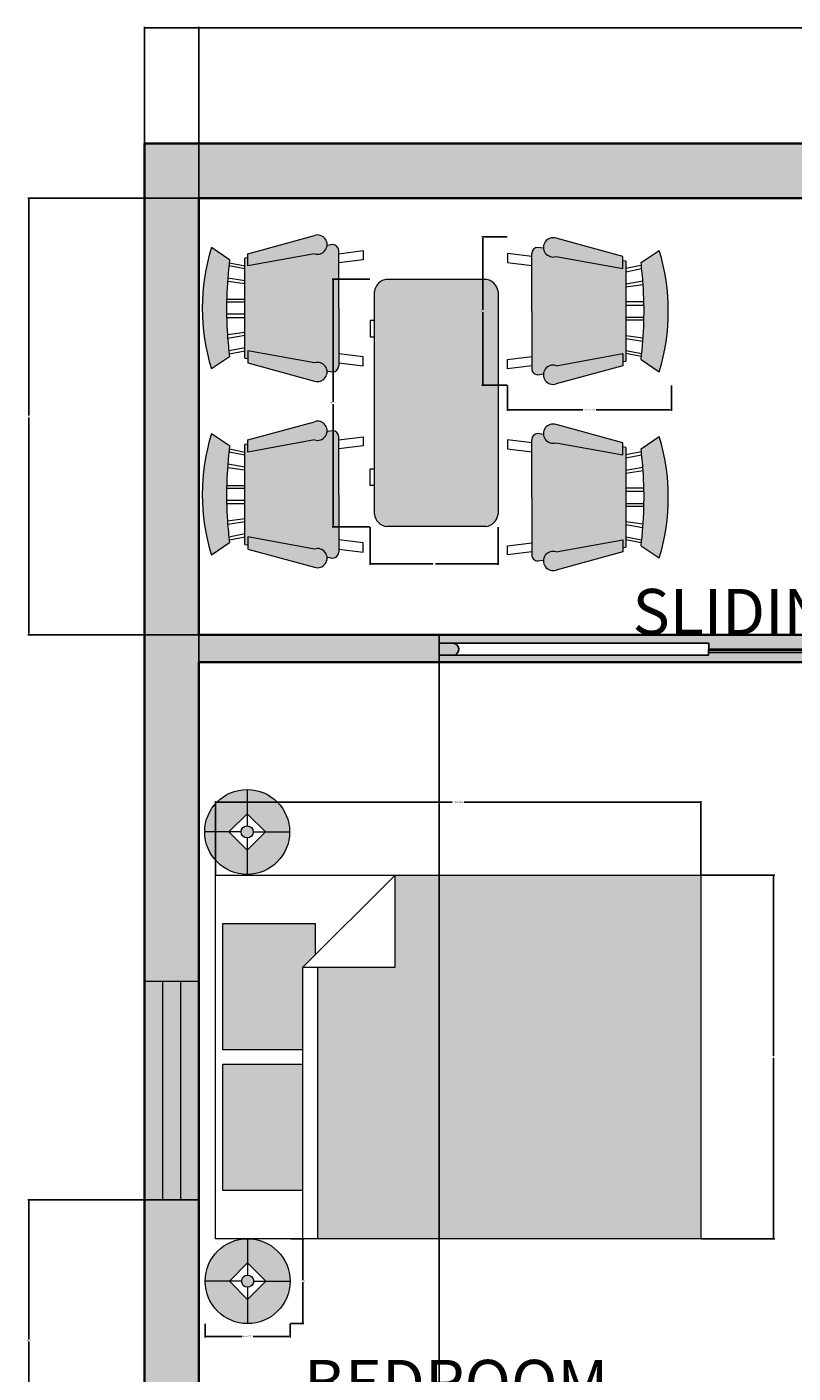
# Model space of a CAD drawing. Units: inches. Extents: x 857 to 1111, y 424 to 822.
# Tile 3 of 9: x 857 to 983, y 600 to 822. Entities that reach past the tile are written whole.
import ezdxf

# ---------------------------------------------------------------- set-up
doc = ezdxf.new("R2010")
doc.units = ezdxf.units.IN
for name, color, linetype, lineweight in [('A-ANNO-DIMS', 2, 'Continuous', 18), ('A-ANNO-TEXT', 7, 'Continuous', 18), ('A-AREA-IDEN', 7, 'Continuous', 25), ('A-DOOR', 3, 'Continuous', 25), ('A-DOOR-PATT', 17, 'Continuous', 13), ('A-FURN', 8, 'Continuous', 18), ('A-FURN-PATT', 9, 'Continuous', 13), ('A-GLAZ', 4, 'Continuous', 18), ('A-GLAZ-PATT', 9, 'Continuous', 13), ('A-WALL', 7, 'Continuous', 35), ('A-WALL-PATT', 252, 'Continuous', 13)]:
    doc.layers.add(name, color=color, linetype=linetype, lineweight=lineweight)
doc.styles.get("Standard").update_dxf_attribs({"font": 'arial.ttf'})
doc.dimstyles.get("Standard").update_dxf_attribs({"dimtxt": 0.18, "dimasz": 0.18, "dimexe": 0.18, "dimexo": 0.0625, "dimgap": 0.09, "dimtad": 0, "dimtih": 1, "dimtoh": 1, "dimdec": 4, "dimzin": 0, "dimdsep": 46, "dimtxsty": 'Standard', "dimcen": 0.09, "dimadec": 0, "dimazin": 0, "dimtfac": 1, "dimtdec": 4, "dimtofl": 0, "dimtmove": 0, "dimatfit": 3, "dimfxl": 1, "dimtolj": 1, "dimtzin": 0, "dimarcsym": 0})

# ---------------------------------------------------------------- blocks, each defined once
blk = doc.blocks.new('Bed - Queen')
for p, q in [((0, -80.00003), (0, 0)), ((0, 0), (59.99999, 0)), ((59.99999, 0), (59.99999, -80.00003)), ((7.99999, -1.2), (28.79998, -1.2)), ((7.99999, -14.4), (7.99999, -1.2)), ((28.79998, -1.2), (28.79998, -14.4)), ((31.19999, -1.2), (51.99999, -1.2)), ((31.19999, -14.4), (31.19999, -1.2)), ((51.99999, -1.2), (51.99999, -16.4)), ((0, -14.4), (44.8, -14.4)), ((59.99999, -29.6), (44.8, -14.4)), ((44.8, -14.4), (44.8, -29.6)), ((44.8, -16.8), (0, -16.8)), ((51.99999, -16.4), (46.79936, -16.4)), ((44.8, -29.6), (59.99999, -29.6)), ((59.99999, -80.00003), (0, -80.00003))]:
    blk.add_line(p, q)
blk = doc.blocks.new('Chair - Rocking')
for p, q in [((-8, -4.5), (-10, -1.5)), ((8, -4.5), (10, -1.5)), ((-6.5, -7), (-7.02225, -4.43)), ((-4.5, -7), (-4.96674, -4.19951)), ((-4, -7), (-4.40532, -4.16272)), ((-1.5, -4.05012), (-1.5, -7)), ((-1, -7), (-1, -4.05012)), ((1, -7), (1, -4.04655)), ((1.5, -4.05012), (1.5, -7)), ((4, -7), (4.40187, -4.18694)), ((4.5, -7), (4.96761, -4.19437)), ((6.5, -7), (7, -4.4057)), ((-7.5, -4.5), (-7, -7)), ((7.5, -4.5), (7, -7)), ((-9, -7.5), (-12, -18.49999)), ((-7, -7.5), (-9, -7.5)), ((-9, -18.49999), (-7, -7.5)), ((-8.23428, -6.99939), (-8.3093, -7.47958)), ((-8.23041, -7), (8.23915, -7)), ((7, -7.5), (9, -7.5)), ((9, -18.49999), (7, -7.5)), ((8.31071, -7.48854), (8.23449, -7.00073)), ((9, -7.5), (12, -18.49999)), ((-10.36644, -20.64523), (-10.5, -21.49999)), ((10.5, -21.49999), (10.3575, -20.58798)), ((-9, -22.49999), (-9.5, -26.49999)), ((0, -22.49999), (-9.5, -22.49999)), ((-8, -26.49999), (-7.5, -22.49999)), ((0, -22.49999), (9.5, -22.49999)), ((8, -26.49999), (7.5, -22.49999)), ((9, -22.49999), (9.5, -26.49999)), ((-9.5, -26.49999), (-8, -26.49999)), ((9.5, -26.49999), (8, -26.49999))]:
    blk.add_line(p, q)
for centre, radius, start, end in [((0, -34.08333), 34.08333, 72.93847, 107.0615), ((0, -68.25004), 64.25, 93.92211, 97.15267), ((0, -68.25004), 64.25, 82.84733, 93.92211), ((-10.5, -18.99999), 1.58114, 161.5651, 18.43495), ((10.5, -18.99999), 1.58114, 161.5651, 18.43495), ((-9.5, -21.49999), 1, 180, 270), ((9.5, -21.49999), 1, 270, 0)]:
    blk.add_arc(centre, radius, start, end)
blk = doc.blocks.new('Desk - 30 x 60 in.')
for p, q in [((-26.999995, 0), (26.999995, 0)), ((-29.999995, -27), (-29.999995, -3)), ((29.999995, -3), (29.999995, -27)), ((26.999995, -30), (-26.999995, -30)), ((-20.000005, -30), (-20.000005, -31)), ((-20.000005, -31), (-16.000005, -31)), ((-16.000005, -31), (-16.000005, -30)), ((15.999995, -31), (15.999995, -30)), ((19.999995, -31), (15.999995, -31)), ((19.999995, -30), (19.999995, -31))]:
    blk.add_line(p, q)
for centre, start, end in [((-26.499995, -3.5), 98.1301, 171.8699), ((26.499995, -3.5), 8.130102, 81.8699), ((-26.499995, -26.5), 188.1301, 261.8699), ((26.499995, -26.5), 278.1301, 351.8699)]:
    blk.add_arc(centre, 3.535534, start, end)
blk = doc.blocks.new('Lamp - Table')
for p, q in [((0, 7), (0, 1)), ((0, 3), (-3, 0)), ((3, 0), (0, 3)), ((-1, 0), (-7, 0)), ((-3, 0), (0, -3)), ((0, -3), (3, 0)), ((1, 0), (7, 0)), ((0, -1), (0, -7))]:
    blk.add_line(p, q)
for radius in [7, 1]:
    blk.add_circle((0, 0), radius)
blk = doc.blocks.new('WIN-36IN-9IN-WALL')
for p, q in [((3, 36), (3, 0)), ((6, 0), (6, 36))]:
    blk.add_line(p, q)
blk.add_lwpolyline([(0, 36), (0, 0), (9, 0), (9, 36)], close=True)
blk = doc.blocks.new('*D18')
at = {"layer": 'A-ANNO-DIMS', "color": 0, "lineweight": -2, "transparency": 16777216}
for p, q in [((936.02, 762.95), (936.02, 758.78)), ((963.02, 762.95), (963.02, 758.78)), ((936.2, 758.96), (948.42, 758.96)), ((962.84, 758.96), (950.62, 758.96))]:
    blk.add_line(p, q, dxfattribs=at)
at = {"layer": 'A-ANNO-DIMS', "color": 0, "transparency": 16777216}
for points in [[(936.2, 758.99), (936.2, 758.93), (936.02, 758.96)], [(962.84, 758.99), (962.84, 758.93), (963.02, 758.96)]]:
    blk.add_solid(points, dxfattribs=at)
at = {"layer": 'Defpoints', "color": 0, "transparency": 16777216}
for p in [(936.02, 763.01), (963.02, 763.01), (963.02, 758.96)]:
    blk.add_point(p, dxfattribs=at)
at = {"layer": 'A-ANNO-DIMS', "color": 0, "transparency": 16777216, "insert": (949.52, 758.96), "char_height": 0.18, "attachment_point": 5}
blk.add_mtext('\\A1;ROCKER 27 TYP.', dxfattribs=at)
blk = doc.blocks.new('*D19')
at = {"layer": 'A-ANNO-DIMS', "color": 0, "lineweight": -2, "transparency": 16777216}
for p, q in [((935.96, 787.45), (931.79, 787.45)), ((931.97, 787.27), (931.97, 775.41)), ((931.97, 763.19), (931.97, 775.05)), ((935.96, 763.01), (931.79, 763.01))]:
    blk.add_line(p, q, dxfattribs=at)
at = {"layer": 'A-ANNO-DIMS', "color": 0, "transparency": 16777216}
for points in [[(931.94, 787.27), (932, 787.27), (931.97, 787.45)], [(931.94, 763.19), (932, 763.19), (931.97, 763.01)]]:
    blk.add_solid(points, dxfattribs=at)
at = {"layer": 'Defpoints', "color": 0, "transparency": 16777216}
for p in [(936.02, 787.45), (931.97, 763.01), (936.02, 763.01)]:
    blk.add_point(p, dxfattribs=at)
at = {"layer": 'A-ANNO-DIMS', "color": 0, "transparency": 16777216, "insert": (931.97, 775.23), "char_height": 0.18, "attachment_point": 5}
blk.add_mtext('\\A1;24 TYP.', dxfattribs=at)
blk = doc.blocks.new('*D22')
at = {"layer": 'A-ANNO-DIMS', "color": 0, "lineweight": -2, "transparency": 16777216}
for p, q in [((886.16, 608.21), (886.16, 605.99)), ((900.16, 608.21), (900.16, 605.99)), ((886.34, 606.17), (892.26, 606.17)), ((899.98, 606.17), (894.06, 606.17))]:
    blk.add_line(p, q, dxfattribs=at)
at = {"layer": 'A-ANNO-DIMS', "color": 0, "transparency": 16777216}
for points in [[(886.34, 606.2), (886.34, 606.14), (886.16, 606.17)], [(899.98, 606.2), (899.98, 606.14), (900.16, 606.17)]]:
    blk.add_solid(points, dxfattribs=at)
at = {"layer": 'Defpoints', "color": 0, "transparency": 16777216}
for p in [(886.16, 608.27), (900.16, 608.27), (900.16, 606.17)]:
    blk.add_point(p, dxfattribs=at)
at = {"layer": 'A-ANNO-DIMS', "color": 0, "transparency": 16777216, "insert": (893.16, 606.17), "char_height": 0.18, "attachment_point": 5}
blk.add_mtext('\\A1;LAMP 14 TYP.', dxfattribs=at)
blk = doc.blocks.new('*D23')
at = {"layer": 'A-ANNO-DIMS', "color": 0, "lineweight": -2, "transparency": 16777216}
for p, q in [((900.23, 622.27), (902.44, 622.27)), ((902.26, 622.09), (902.26, 615.45)), ((902.26, 608.45), (902.26, 615.09)), ((900.23, 608.27), (902.44, 608.27))]:
    blk.add_line(p, q, dxfattribs=at)
at = {"layer": 'A-ANNO-DIMS', "color": 0, "transparency": 16777216}
for points in [[(902.23, 622.09), (902.29, 622.09), (902.26, 622.27)], [(902.23, 608.45), (902.29, 608.45), (902.26, 608.27)]]:
    blk.add_solid(points, dxfattribs=at)
at = {"layer": 'Defpoints', "color": 0, "transparency": 16777216}
for p in [(900.16, 622.27), (902.26, 622.27), (900.16, 608.27)]:
    blk.add_point(p, dxfattribs=at)
at = {"layer": 'A-ANNO-DIMS', "color": 0, "transparency": 16777216, "insert": (902.26, 615.27), "char_height": 0.18, "attachment_point": 5}
blk.add_mtext('\\A1;14 TYP.', dxfattribs=at)
blk = doc.blocks.new('*D28')
at = {"layer": 'A-ANNO-DIMS', "color": 0, "lineweight": -2, "transparency": 16777216}
for p, q in [((887.88, 682.29), (887.88, 694.41)), ((888.06, 694.23), (926.89, 694.23)), ((967.7, 694.23), (928.88, 694.23)), ((967.88, 682.29), (967.88, 694.41))]:
    blk.add_line(p, q, dxfattribs=at)
at = {"layer": 'A-ANNO-DIMS', "color": 0, "transparency": 16777216}
for points in [[(888.06, 694.26), (888.06, 694.2), (887.88, 694.23)], [(967.7, 694.26), (967.7, 694.2), (967.88, 694.23)]]:
    blk.add_solid(points, dxfattribs=at)
at = {"layer": 'Defpoints', "color": 0, "transparency": 16777216}
for p in [(887.88, 694.23), (887.88, 682.23), (967.88, 682.23)]:
    blk.add_point(p, dxfattribs=at)
at = {"layer": 'A-ANNO-DIMS', "color": 0, "transparency": 16777216, "insert": (927.88, 694.23), "char_height": 0.18, "attachment_point": 5}
blk.add_mtext('\\A1;QUEEN BED 80', dxfattribs=at)
blk = doc.blocks.new('*D29')
at = {"layer": 'A-ANNO-DIMS', "color": 0, "lineweight": -2, "transparency": 16777216}
for p, q in [((967.95, 682.23), (980.06, 682.23)), ((979.88, 682.05), (979.88, 652.41)), ((979.88, 622.41), (979.88, 652.04)), ((967.95, 622.23), (980.06, 622.23))]:
    blk.add_line(p, q, dxfattribs=at)
at = {"layer": 'A-ANNO-DIMS', "color": 0, "transparency": 16777216}
for points in [[(979.85, 682.05), (979.91, 682.05), (979.88, 682.23)], [(979.85, 622.41), (979.91, 622.41), (979.88, 622.23)]]:
    blk.add_solid(points, dxfattribs=at)
at = {"layer": 'Defpoints', "color": 0, "transparency": 16777216}
for p in [(967.88, 682.23), (979.88, 682.23), (967.88, 622.23)]:
    blk.add_point(p, dxfattribs=at)
at = {"layer": 'A-ANNO-DIMS', "color": 0, "transparency": 16777216, "insert": (979.88, 652.23), "char_height": 0.18, "attachment_point": 5}
blk.add_mtext('\\A1;60', dxfattribs=at)
blk = doc.blocks.new('*D42')
at = {"layer": 'A-ANNO-DIMS', "color": 0, "lineweight": -2, "transparency": 16777216}
for p, q in [((913.32, 780.49), (907.08, 780.49)), ((907.26, 780.31), (907.26, 760.27)), ((907.26, 739.86), (907.26, 759.9)), ((913.32, 739.68), (907.08, 739.68))]:
    blk.add_line(p, q, dxfattribs=at)
at = {"layer": 'A-ANNO-DIMS', "color": 0, "transparency": 16777216}
for points in [[(907.23, 780.31), (907.29, 780.31), (907.26, 780.49)], [(907.23, 739.86), (907.29, 739.86), (907.26, 739.68)]]:
    blk.add_solid(points, dxfattribs=at)
at = {"layer": 'Defpoints', "color": 0, "transparency": 16777216}
for p in [(913.38, 780.49), (907.26, 739.68), (913.38, 739.68)]:
    blk.add_point(p, dxfattribs=at)
at = {"layer": 'A-ANNO-DIMS', "color": 0, "transparency": 16777216, "insert": (907.26, 760.09), "char_height": 0.18, "attachment_point": 5}
blk.add_mtext('\\A1;DESK 41', dxfattribs=at)
blk = doc.blocks.new('*D43')
at = {"layer": 'A-ANNO-DIMS', "color": 0, "lineweight": -2, "transparency": 16777216}
for p, q in [((913.38, 739.62), (913.38, 733.38)), ((934.46, 739.62), (934.46, 733.38)), ((913.56, 733.56), (923.72, 733.56)), ((934.28, 733.56), (924.12, 733.56))]:
    blk.add_line(p, q, dxfattribs=at)
at = {"layer": 'A-ANNO-DIMS', "color": 0, "transparency": 16777216}
for points in [[(913.56, 733.59), (913.56, 733.53), (913.38, 733.56)], [(934.28, 733.59), (934.28, 733.53), (934.46, 733.56)]]:
    blk.add_solid(points, dxfattribs=at)
at = {"layer": 'Defpoints', "color": 0, "transparency": 16777216}
for p in [(913.38, 739.68), (934.46, 739.68), (934.46, 733.56)]:
    blk.add_point(p, dxfattribs=at)
at = {"layer": 'A-ANNO-DIMS', "color": 0, "transparency": 16777216, "insert": (923.92, 733.56), "char_height": 0.18, "attachment_point": 5}
blk.add_mtext('\\A1;21', dxfattribs=at)
blk = doc.blocks.new('*D44')
at = {"layer": 'A-ANNO-DIMS', "color": 0, "lineweight": -2, "transparency": 16777216}
for p, q in [((876.14, 802.92), (876.14, 822.09)), ((876.32, 821.91), (983.85, 821.91)), ((1091.96, 821.91), (984.43, 821.91)), ((1092.14, 802.92), (1092.14, 822.09))]:
    blk.add_line(p, q, dxfattribs=at)
at = {"layer": 'A-ANNO-DIMS', "color": 0, "transparency": 16777216}
for points in [[(876.32, 821.94), (876.32, 821.88), (876.14, 821.91)], [(1091.96, 821.94), (1091.96, 821.88), (1092.14, 821.91)]]:
    blk.add_solid(points, dxfattribs=at)
at = {"layer": 'Defpoints', "color": 0, "transparency": 16777216}
for p in [(1092.14, 821.91), (876.14, 802.86), (1092.14, 802.86)]:
    blk.add_point(p, dxfattribs=at)
at = {"layer": 'A-ANNO-DIMS', "color": 0, "transparency": 16777216, "insert": (984.14, 821.91), "char_height": 0.18, "attachment_point": 5}
blk.add_mtext('\\A1;216', dxfattribs=at)
blk = doc.blocks.new('*D48')
at = {"layer": 'A-ANNO-DIMS', "color": 0, "lineweight": -2, "transparency": 16777216}
for p, q in [((885.14, 582.42), (885.14, 822.09)), ((885.32, 821.91), (935, 821.91)), ((985.46, 821.91), (935.77, 821.91)), ((985.64, 582.42), (985.64, 822.09))]:
    blk.add_line(p, q, dxfattribs=at)
at = {"layer": 'A-ANNO-DIMS', "color": 0, "transparency": 16777216}
for points in [[(885.32, 821.94), (885.32, 821.88), (885.14, 821.91)], [(985.46, 821.94), (985.46, 821.88), (985.64, 821.91)]]:
    blk.add_solid(points, dxfattribs=at)
at = {"layer": 'Defpoints', "color": 0, "transparency": 16777216}
for p in [(985.64, 821.91), (885.14, 582.36), (985.64, 582.36)]:
    blk.add_point(p, dxfattribs=at)
at = {"layer": 'A-ANNO-DIMS', "color": 0, "transparency": 16777216, "insert": (935.39, 821.91), "char_height": 0.18, "attachment_point": 5}
blk.add_mtext('\\A1;100.5', dxfattribs=at)
blk = doc.blocks.new('*D54')
at = {"layer": 'A-ANNO-DIMS', "color": 0, "lineweight": -2, "transparency": 16777216}
for p, q in [((885.07, 793.86), (856.91, 793.86)), ((857.09, 793.68), (857.09, 758.04)), ((857.09, 722.04), (857.09, 757.68)), ((885.07, 721.86), (856.91, 721.86))]:
    blk.add_line(p, q, dxfattribs=at)
at = {"layer": 'A-ANNO-DIMS', "color": 0, "transparency": 16777216}
for points in [[(857.06, 793.68), (857.12, 793.68), (857.09, 793.86)], [(857.06, 722.04), (857.12, 722.04), (857.09, 721.86)]]:
    blk.add_solid(points, dxfattribs=at)
at = {"layer": 'Defpoints', "color": 0, "transparency": 16777216}
for p in [(857.09, 793.86), (885.14, 793.86), (885.14, 721.86)]:
    blk.add_point(p, dxfattribs=at)
at = {"layer": 'A-ANNO-DIMS', "color": 0, "transparency": 16777216, "insert": (857.09, 757.86), "char_height": 0.18, "attachment_point": 5}
blk.add_mtext('\\A1;72', dxfattribs=at)
blk = doc.blocks.new('*D56')
at = {"layer": 'A-ANNO-DIMS', "color": 0, "lineweight": -2, "transparency": 16777216}
for p, q in [((924.77, 717.29), (924.77, 423.63)), ((1053.97, 717.29), (1053.97, 423.63)), ((924.95, 423.81), (988.99, 423.81)), ((1053.79, 423.81), (989.75, 423.81))]:
    blk.add_line(p, q, dxfattribs=at)
at = {"layer": 'A-ANNO-DIMS', "color": 0, "transparency": 16777216}
for points in [[(924.95, 423.84), (924.95, 423.78), (924.77, 423.81)], [(1053.79, 423.84), (1053.79, 423.78), (1053.97, 423.81)]]:
    blk.add_solid(points, dxfattribs=at)
at = {"layer": 'Defpoints', "color": 0, "transparency": 16777216}
for p in [(924.77, 717.36), (1053.97, 717.36), (1053.97, 423.81)]:
    blk.add_point(p, dxfattribs=at)
at = {"layer": 'A-ANNO-DIMS', "color": 0, "transparency": 16777216, "insert": (989.37, 423.81), "char_height": 0.18, "attachment_point": 5}
blk.add_mtext('\\A1;129.2', dxfattribs=at)
blk = doc.blocks.new('*D59')
at = {"layer": 'A-ANNO-DIMS', "color": 0, "lineweight": -2, "transparency": 16777216}
for p, q in [((885.07, 628.69), (856.91, 628.69)), ((857.09, 628.51), (857.09, 605.7)), ((857.09, 582.54), (857.09, 605.34)), ((885.07, 582.36), (856.91, 582.36))]:
    blk.add_line(p, q, dxfattribs=at)
at = {"layer": 'A-ANNO-DIMS', "color": 0, "transparency": 16777216}
for points in [[(857.06, 628.51), (857.12, 628.51), (857.09, 628.69)], [(857.06, 582.54), (857.12, 582.54), (857.09, 582.36)]]:
    blk.add_solid(points, dxfattribs=at)
at = {"layer": 'Defpoints', "color": 0, "transparency": 16777216}
for p in [(857.09, 628.69), (885.14, 628.69), (885.14, 582.36)]:
    blk.add_point(p, dxfattribs=at)
at = {"layer": 'A-ANNO-DIMS', "color": 0, "transparency": 16777216, "insert": (857.09, 605.52), "char_height": 0.18, "attachment_point": 5}
blk.add_mtext('\\A1;46.33', dxfattribs=at)

msp = doc.modelspace()

# ---------------------------------------------------------------- hatches: boundary and pattern name
at = {"layer": 'A-DOOR-PATT'}
h = msp.add_hatch(color=256, dxfattribs=at)
h.dxf.hatch_style = 1
h.set_gradient(color1=(0, 0, 255), color2=(255, 255, 0))
h.paths.add_polyline_path([(1053.9717, 718.9594), (969.1676, 718.9594), (969.1596, 718.4668), (927.0274, 718.4668), (924.7696, 718.4668), (924.7696, 717.3567), (1053.9717, 717.3567)], flags=17)
h.paths.add_polyline_path([(969.1676, 718.9594), (969.1922, 720.4869), (927.0274, 720.4869, -0.93409348), (927.0274, 718.4668), (969.1596, 718.4668)], flags=0)
h.paths.add_polyline_path([(1053.9717, 721.8567), (924.7696, 721.8567), (924.7696, 720.4869), (926.8896, 720.4869, -0.03407618), (927.0274, 720.4869), (927.0302, 720.4869), (969.1922, 720.4869), (969.1759, 719.4769), (1053.9717, 719.4769)], flags=17)
h.paths.add_polyline_path([(1053.9717, 721.8567), (924.7696, 721.8567), (924.7696, 717.3567), (1053.9717, 717.3567)])
h.paths.add_polyline_path([(969.1596, 718.4668), (927.0274, 718.4668, 0.93409348), (927.0274, 720.4869), (969.1922, 720.4869)], flags=16)
h = msp.add_hatch(color=256, dxfattribs=at)
h.dxf.hatch_style = 1
h.set_gradient(color1=(0, 0, 255), color2=(255, 255, 0), name='INVCYLINDER')
h.paths.add_polyline_path([(1053.9717, 721.8567), (924.7696, 721.8567), (924.7696, 720.4869), (927.0302, 720.4869), (969.1922, 720.4869), (969.1759, 719.4769), (1053.9717, 719.4769)], flags=17)
h.paths.add_polyline_path([(1053.9717, 718.9594), (969.1676, 718.9594), (969.1759, 719.4769), (1053.9717, 719.4769), (1053.9717, 721.8567), (924.7696, 721.8567), (924.7696, 717.3567), (1053.9717, 717.3567)])
h.paths.add_polyline_path([(969.1596, 718.4668), (927.0274, 718.4668, 0.93409348), (927.0274, 720.4869), (969.1922, 720.4869)], flags=16)
h = msp.add_hatch(color=256, dxfattribs=at)
h.dxf.hatch_style = 1
h.set_gradient(color1=(0, 0, 255), color2=(255, 255, 0), name='SPHERICAL')
h.paths.add_polyline_path([(1053.9717, 721.8567), (924.7696, 721.8567), (924.7696, 717.3567), (1053.9717, 717.3567), (1053.9717, 718.9594), (969.1676, 718.9594), (969.1759, 719.4769), (1053.9717, 719.4769)])
h.paths.add_polyline_path([(927.0274, 720.4869, -0.93409348), (927.0274, 718.4668), (969.1596, 718.4668), (969.1922, 720.4869)], flags=16)
at = {"layer": 'A-FURN-PATT'}
h = msp.add_hatch(color=256, dxfattribs=at)
h.dxf.hatch_style = 1
h.paths.add_polyline_path([(967.884, 682.2251), (917.484, 682.2251), (917.484, 667.0251), (904.684, 667.0251), (904.684, 622.2251), (967.884, 622.2251)])
h.paths.add_polyline_path([(902.284, 667.0251), (904.284, 669.0251), (904.284, 674.2251), (889.084, 674.2251), (889.084, 653.4251), (902.284, 653.4251)])
h.paths.add_polyline_path([(902.284, 651.0251), (889.084, 651.0251), (889.084, 630.2251), (902.284, 630.2251)])
h.paths.add_polyline_path([(904.1909, 787.6962), (893.1909, 784.6962), (893.1909, 782.6962), (904.1909, 784.6962, 1.38742744)])
h.paths.add_polyline_path([(904.1909, 766.6962), (893.1909, 768.6962), (893.1909, 766.6962), (904.1909, 763.6962, 1.38742744)])
h.paths.add_polyline_path([(889.8414, 771.3015, -0.04836039), (890.1909, 783.6962), (887.1909, 785.6962, 0.15000001), (887.1909, 765.6962), (890.1909, 767.6962, -0.01409681)])
h.paths.add_polyline_path([(904.1909, 753.9927, 1.38742744), (904.1909, 756.9927), (893.1909, 753.9927), (893.1909, 751.9927)])
h.paths.add_polyline_path([(904.1909, 735.9927), (893.1909, 737.9927), (893.1909, 735.9927), (904.1909, 732.9927, 1.38742744)])
h.paths.add_polyline_path([(890.1909, 752.9927), (887.1909, 754.9927, 0.15000001), (887.1909, 734.9927), (890.1909, 736.9928, -0.01409681), (889.8414, 740.598, -0.04836039)])
h.paths.add_polyline_path([(955.0194, 737.5254), (944.0194, 735.5254, 1.38742744), (944.0194, 732.5254), (955.0194, 735.5254)])
h.paths.add_polyline_path([(955.0194, 753.5254), (944.0194, 756.5254, 1.38742744), (944.0194, 753.5254), (955.0194, 751.5254)])
h.paths.add_polyline_path([(955.0194, 766.2288), (955.0194, 768.2288), (944.0194, 766.2288, 1.38742744), (944.0194, 763.2288)])
h.paths.add_polyline_path([(955.0194, 784.2288), (944.0194, 787.2288, 1.38742744), (944.0194, 784.2288), (955.0194, 782.2288)])
h.paths.add_polyline_path([(961.0194, 785.2288), (958.0194, 783.2288, -0.01409681), (958.3689, 779.6235, -0.04836039), (958.0194, 767.2289), (961.0194, 765.2288, 0.15000001)])
h.paths.add_polyline_path([(961.0194, 754.5254), (958.0194, 752.5254, -0.01409681), (958.3689, 748.9201, -0.04836039), (958.0194, 736.5254), (961.0194, 734.5254, 0.15000001)])
h = msp.add_hatch(color=256, dxfattribs=at)
h.dxf.hatch_style = 1
h.paths.add_polyline_path([(908.1909, 744.9927), (908.1909, 754.4927, 0.41421356), (907.1909, 755.4927), (906.2654, 755.3481, -0.48335183), (904.1909, 753.9927), (893.1909, 751.9927), (893.1909, 753.3052), (892.6909, 753.2271), (892.6909, 736.7584), (893.1909, 736.6802), (893.1909, 737.9927), (904.1909, 735.9927, -0.4833507), (906.2654, 734.6373), (907.1909, 734.4927, 0.41421356), (908.1909, 735.4927)])
h.paths.add_polyline_path([(908.1909, 785.1962, 0.41421356), (907.1909, 786.1962), (906.2654, 786.0516, -0.48335183), (904.1909, 784.6962), (893.1909, 782.6962), (893.1909, 784.0087), (892.6909, 783.9306), (892.6909, 767.4618), (893.1909, 767.3837), (893.1909, 768.6962), (904.1909, 766.6962, -0.4833507), (906.2654, 765.3408), (907.1909, 765.1962, 0.41421356), (908.1909, 766.1962), (908.1909, 775.6962)])
h.paths.add_polyline_path([(955.5194, 783.4632), (955.0194, 783.5413), (955.0194, 782.2288), (944.0194, 784.2288, -0.4833507), (941.9449, 785.5842), (941.0194, 785.7288, 0.41421356), (940.0194, 784.7288), (940.0194, 775.2288), (940.0194, 765.7288, 0.41421356), (941.0194, 764.7288), (941.9449, 764.8734, -0.48335183), (944.0194, 766.2288), (955.0194, 768.2288), (955.0194, 766.9163), (955.5194, 766.9945)])
h.paths.add_polyline_path([(955.5194, 752.7598), (955.0194, 752.8379), (955.0194, 751.5254), (944.0194, 753.5254, -0.4833507), (941.9449, 754.8808), (941.0194, 755.0254, 0.41421356), (940.0194, 754.0254), (940.0194, 744.5254), (940.0194, 735.0254, 0.41421356), (941.0194, 734.0254), (941.9449, 734.17, -0.48335183), (944.0194, 735.5254), (955.0194, 737.5254), (955.0194, 736.2129), (955.5194, 736.291)])
h = msp.add_hatch(color=256, dxfattribs=at)
h.dxf.hatch_style = 1
h.set_gradient(color1=(0, 0, 255), color2=(255, 255, 0), name='INVSPHERICAL')
h.paths.add_polyline_path([(934.4613, 778.448, 0.33333323), (932.421, 780.4883), (916.0987, 780.4883, 0.33333323), (914.0584, 778.448), (914.0584, 741.7229, 0.33333323), (916.0987, 739.6826), (932.421, 739.6826, 0.33333323), (934.4613, 741.7229)])
h = msp.add_hatch(color=256, dxfattribs=at)
h.dxf.hatch_style = 1
h.paths.add_polyline_path([(893.0912, 692.3455), (893.0912, 696.3455, 0.41421356), (886.0912, 689.3455), (890.0912, 689.3455)])
h.paths.add_polyline_path([(890.0912, 689.3455), (886.0912, 689.3455, 0.41421356), (893.0912, 682.3455), (893.0912, 686.3455)])
h.paths.add_polyline_path([(900.0912, 689.3455), (896.0912, 689.3455), (893.0912, 686.3455), (893.0912, 682.3455, 0.41421356)])
h.paths.add_polyline_path([(893.0912, 696.3455), (893.0912, 692.3455), (896.0912, 689.3455), (900.0912, 689.3455, 0.41421356)])
h.paths.add_polyline_path([(892.0912, 689.3455, 1), (894.0912, 689.3455, 1)])
h.paths.add_polyline_path([(893.9715, 622.2251), (893.1628, 622.2251), (893.1628, 618.272), (896.1628, 615.272), (900.1628, 615.272, 0.38069507)])
h.paths.add_polyline_path([(893.1628, 618.272), (893.1628, 622.2251), (892.3542, 622.2251, 0.38069507), (886.1628, 615.272), (890.1628, 615.272)])
h.paths.add_polyline_path([(893.1628, 612.272), (890.1628, 615.272), (886.1628, 615.272, 0.41421356), (893.1628, 608.272)])
h.paths.add_polyline_path([(900.1628, 615.272), (896.1628, 615.272), (893.1628, 612.272), (893.1628, 608.272, 0.41421356)])
h.paths.add_polyline_path([(892.1628, 615.272, 1), (894.1628, 615.272, 1)])
at = {"layer": 'A-GLAZ-PATT'}
h = msp.add_hatch(color=256, dxfattribs=at)
h.dxf.hatch_style = 1
h.set_gradient(color1=(0, 0, 255), color2=(255, 255, 0))
h.paths.add_polyline_path([(885.1369, 664.6868), (882.1369, 664.6868), (882.1369, 628.6868), (885.1369, 628.6868)])
h.paths.add_polyline_path([(882.1369, 664.6868), (879.1369, 664.6868), (879.1369, 628.6868), (882.1369, 628.6868)])
h.paths.add_polyline_path([(879.1369, 664.6868), (876.1369, 664.6868), (876.1369, 628.6868), (879.1369, 628.6868)])
at = {"layer": 'A-WALL-PATT'}
h = msp.add_hatch(color=256, dxfattribs=at)
h.dxf.hatch_style = 1
h.paths.add_polyline_path([(924.7696, 721.8567), (885.1369, 721.8567), (885.1369, 793.8567), (1083.1369, 793.8567), (1083.1369, 721.8567), (1053.9717, 721.8567), (1053.9717, 717.3567), (1083.1369, 717.3567), (1083.1369, 706.6069), (1092.1369, 706.6069), (1092.1369, 802.8567), (876.1369, 802.8567), (876.1369, 664.6868), (885.1369, 664.6868), (885.1369, 717.3567), (924.7696, 717.3567)])
h.paths.add_polyline_path([(985.6369, 582.3567), (885.1369, 582.3567), (885.1369, 585.1154), (885.1369, 628.6868), (876.1369, 628.6868), (876.1369, 529.0363), (885.1369, 529.0363), (885.1369, 577.8567), (981.1369, 577.8567), (985.6369, 577.8567)])
h.paths.add_polyline_path([(885.1369, 493.0363), (876.1369, 493.0363), (876.1369, 442.8567), (991.6369, 442.8567), (991.6369, 451.8567), (985.6369, 451.8567), (985.6369, 535.8567), (981.1369, 535.8567), (981.1369, 451.8567), (885.1369, 451.8567)])
h.paths.add_polyline_path([(1092.1369, 553.8025), (1083.1369, 553.8025), (1083.1369, 451.8567), (1030.6369, 451.8567), (1027.6369, 451.8567), (1027.6369, 442.8567), (1092.1369, 442.8567)])
h.paths.add_polyline_path([(1092.1369, 670.6069), (1083.1369, 670.6069), (1083.1369, 662.5384, -0.02676862), (1083.1369, 657.4501), (1083.1369, 589.8025), (1092.1369, 589.8025)])

# ---------------------------------------------------------------- linework, layer by layer
at = {"layer": 'A-DOOR'}
for p, q in [((924.7696, 720.4869), (927.0302, 720.4869)), ((927.0274, 720.4869), (969.1922, 720.4869)), ((969.1596, 718.4668), (969.1922, 720.4869)), ((969.1734, 719.3176), (1053.9717, 719.3176)), ((969.1759, 719.4769), (1053.9717, 719.4769)), ((924.7696, 718.4668), (927.0274, 718.4668)), ((927.0274, 718.4668), (969.1596, 718.4668)), ((969.1676, 718.9594), (1053.9717, 718.9594))]:
    msp.add_line(p, q, dxfattribs=at)
msp.add_lwpolyline([(924.7696, 721.8567), (1053.9717, 721.8567), (1053.9717, 717.3567), (924.7696, 717.3567)], close=True, dxfattribs=at)
msp.add_arc((926.9585, 719.4769), 1.0124, 273.903332, 93.903332, dxfattribs=at)
at = {"layer": 'A-WALL'}
for p, q in [((1083.1369, 793.8567), (885.1369, 793.8567)), ((885.1369, 793.8567), (885.1369, 721.8567)), ((1083.1369, 721.8567), (885.1369, 721.8567)), ((1083.1369, 717.3567), (885.1369, 717.3567)), ((885.1369, 717.3567), (885.1369, 582.3567))]:
    msp.add_line(p, q, dxfattribs=at)
msp.add_lwpolyline([(1027.6369, 442.8567), (1092.1369, 442.8567), (1092.1369, 802.8567), (876.1369, 802.8567), (876.1369, 442.8567), (991.6369, 442.8567)], dxfattribs=at)

# ---------------------------------------------------------------- block references
at = {"layer": 'A-FURN'}
for name, p, rotation in [('Chair - Rocking', (885.6909, 775.6962), 90), ('Chair - Rocking', (962.5194, 775.2288), 270), ('Chair - Rocking', (885.6909, 744.9927), 90), ('Chair - Rocking', (962.5194, 744.5254), 270), ('Bed - Queen', (887.884, 622.2251), 90)]:
    msp.add_blockref(name, p, dxfattribs=dict(at, rotation=rotation))
at = {"layer": 'A-FURN', "xscale": 0.6800963287183404, "yscale": 0.6800963287183404, "zscale": 0.6800963287183404, "rotation": 270}
msp.add_blockref('Desk - 30 x 60 in.', (934.4613, 760.0855), dxfattribs=at)
at = {"layer": 'A-FURN'}
for p in [(893.0912, 689.3455), (893.1628, 615.272)]:
    msp.add_blockref('Lamp - Table', p, dxfattribs=at)
at = {"layer": 'A-GLAZ'}
msp.add_blockref('WIN-36IN-9IN-WALL', (876.1369, 628.6868), dxfattribs=at)

# ---------------------------------------------------------------- texts
at = {"layer": 'A-ANNO-TEXT'}
msp.add_text('SLIDING DOOR ', height=7.55928, dxfattribs=at).set_placement((956.6211, 721.8567))
at = {"layer": 'A-AREA-IDEN'}
msp.add_text('BEDROOM ', height=7.55928, dxfattribs=at).set_placement((902.4461, 594.7313))

# ---------------------------------------------------------------- dimensions: what is measured, and where the dimension line sits
at = {"layer": 'A-ANNO-DIMS'}
for base, p1, p2, override, picture, middle in [((1092.1369, 821.9067), (876.1369, 802.8567), (1092.1369, 802.8567), {"dimdec": 0, "dimlfac": 1, "dimrnd": 0, "dimzin": 0, "dimdsep": 46, "dimlunit": 2}, '*D44', (984.1369, 821.9067)), ((985.6369, 821.9067), (885.1369, 582.3567), (985.6369, 582.3567), {"dimdec": 1, "dimlfac": 1, "dimrnd": 0, "dimzin": 0, "dimdsep": 46, "dimlunit": 2}, '*D48', (935.3869, 821.9067)), ((934.4613, 733.5617), (913.3783, 739.6826), (934.4613, 739.6826), {"dimdec": 0, "dimlfac": 1, "dimrnd": 0, "dimzin": 0, "dimdsep": 46, "dimlunit": 2}, '*D43', (923.9198, 733.5617)), ((1053.9717, 423.8067), (924.7696, 717.3567), (1053.9717, 717.3567), {"dimdec": 1, "dimlfac": 1, "dimrnd": 0, "dimzin": 0, "dimdsep": 46, "dimlunit": 2}, '*D56', (989.3707, 423.8067))]:
    dim = msp.add_linear_dim(base=base, p1=p1, p2=p2, dimstyle='Standard', override=override, dxfattribs=at)
    dim.commit()
    dim.dimension.update_dxf_attribs({"geometry": picture, "text_midpoint": middle})
for base, p1, p2, override, picture, middle in [((857.0869, 793.8567), (885.1369, 721.8567), (885.1369, 793.8567), {"dimdec": 0, "dimlfac": 1, "dimrnd": 0, "dimzin": 0, "dimdsep": 46, "dimlunit": 2}, '*D54', (857.0869, 757.8567)), ((979.884, 682.2251), (967.884, 622.2251), (967.884, 682.2251), {"dimdec": 0, "dimlfac": 1, "dimrnd": 0, "dimzin": 0, "dimdsep": 46, "dimlunit": 2}, '*D29', (979.884, 652.2251)), ((857.0869, 628.6868), (885.1369, 582.3567), (885.1369, 628.6868), {"dimdec": 2, "dimlfac": 1, "dimrnd": 0, "dimzin": 0, "dimdsep": 46, "dimlunit": 2}, '*D59', (857.0869, 605.5217))]:
    dim = msp.add_linear_dim(base=base, p1=p1, p2=p2, angle=90, dimstyle='Standard', override=override, dxfattribs=at)
    dim.commit()
    dim.dimension.update_dxf_attribs({"geometry": picture, "text_midpoint": middle})
for base, p1, p2, angle, text, picture, middle in [((931.9694, 763.0113), (936.0194, 787.4464), (936.0194, 763.0113), 270, '<> TYP.', '*D19', (931.9694, 775.2288)), ((907.2575, 739.6826), (913.3783, 780.4883), (913.3783, 739.6826), 270, 'DESK <>', '*D42', (907.2575, 760.0855)), ((887.884, 694.2251), (967.884, 682.2251), (887.884, 682.2251), 180, 'QUEEN BED <>', '*D28', (927.884, 694.2251)), ((902.2628, 622.272), (900.1628, 608.272), (900.1628, 622.272), 90, '<> TYP.', '*D23', (902.2628, 615.272))]:
    dim = msp.add_linear_dim(base=base, p1=p1, p2=p2, angle=angle, text=text, dimstyle='Standard', override={"dimdec": 0, "dimlfac": 1, "dimrnd": 0, "dimzin": 0, "dimdsep": 46, "dimlunit": 2}, dxfattribs=at)
    dim.commit()
    dim.dimension.update_dxf_attribs({"geometry": picture, "text_midpoint": middle})
for base, p1, p2, text, picture, middle in [((963.0194, 758.9613), (936.0194, 763.0113), (963.0194, 763.0113), 'ROCKER <> TYP.', '*D18', (949.5194, 758.9613)), ((900.1628, 606.172), (886.1628, 608.272), (900.1628, 608.272), 'LAMP <> TYP.', '*D22', (893.1628, 606.172))]:
    dim = msp.add_linear_dim(base=base, p1=p1, p2=p2, text=text, dimstyle='Standard', override={"dimdec": 0, "dimlfac": 1, "dimrnd": 0, "dimzin": 0, "dimdsep": 46, "dimlunit": 2}, dxfattribs=at)
    dim.commit()
    dim.dimension.update_dxf_attribs({"geometry": picture, "text_midpoint": middle})

doc.saveas('drawing.dxf')
